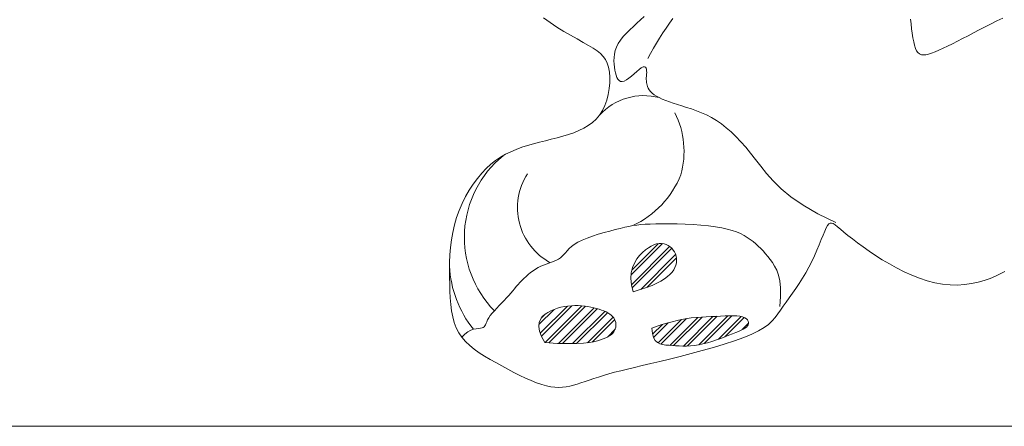
# Model space of a CAD drawing. Units: inches. Extents: x -17 to 1735, y -531 to 60.
# Tile 7 of 27: x 1734.668631 to 1734.675388, y -150.224179 to -150.221388. Entities that reach past the tile are written whole.
import ezdxf

# ---------------------------------------------------------------- set-up
doc = ezdxf.new("R2010")
doc.units = ezdxf.units.IN
doc.header["$MEASUREMENT"] = 0
doc.layers.add('A-FURN', color=242, linetype='Continuous', lineweight=18, true_color=0xcd2027)

# ---------------------------------------------------------------- blocks, each defined once
blk = doc.blocks.new('childrens_room_2')
for p, q in [((70.09560985742021, 54.02979216459647), (70.09445746645682, 54.03061162945817)), ((70.11141095916858, 54.03028320464222), (70.11203336932115, 54.03085697882346)), ((70.11702802801622, 54.03048828868344), (70.11644430215122, 54.02968633954009)), ((70.15854766663281, 54.02956733155446), (70.15844540531864, 54.03041195851841)), ((70.17456501944574, 54.03058353331147), (70.17352318415536, 54.03007965674482)), ((70.09680749046268, 54.02901020311986), (70.09560985742021, 54.02979216459647)), ((70.09801667475725, 54.02827055314123), (70.09680749046268, 54.02901020311986)), ((70.10951143574087, 54.02853423031633), (70.11013384589344, 54.02912183038137)), ((70.11013384589344, 54.02912183038137), (70.11077240256012, 54.02970482181848)), ((70.11077240256012, 54.02970482181848), (70.11141095916858, 54.03028320464222)), ((70.11585971132038, 54.02885184196787), (70.115280310401, 54.0279914208499)), ((70.11644430215122, 54.02968633954009), (70.11585971132038, 54.02885184196787)), ((70.15864992794698, 54.02873307398698), (70.15854766663281, 54.02956733155446)), ((70.15875680256752, 54.02792589209861), (70.15864992794698, 54.02873307398698)), ((70.17145796674188, 54.02904886050095), (70.17044381123154, 54.02853115807232)), ((70.17248596217135, 54.02956656293685), (70.17145796674188, 54.02904886050095)), ((70.17352318415536, 54.03007965674482), (70.17248596217135, 54.02956656293685)), ((70.09920371930232, 54.02757802278796), (70.09801667475725, 54.02827055314123)), ((70.10033493315453, 54.02693742018749), (70.09920371930232, 54.02757802278796)), ((70.10137662531227, 54.02635355346723), (70.10033493315453, 54.02693742018749)), ((70.10790254979977, 54.02674377838997), (70.10837964120904, 54.02734520431699)), ((70.10837964120904, 54.02734520431699), (70.1089213186747, 54.02794202162334)), ((70.1089213186747, 54.02794202162334), (70.10951143574087, 54.02853423031633)), ((70.11471215444502, 54.02711170109109), (70.11416129827151, 54.02621930758908)), ((70.115280310401, 54.0279914208499), (70.11471215444502, 54.02711170109109)), ((70.15887290380081, 54.02716249216467), (70.15875680256752, 54.02792589209861)), ((70.15900284489501, 54.02645958046054), (70.15887290380081, 54.02716249216467)), ((70.16753061291413, 54.02702432905647), (70.1666186226171, 54.02655405706031)), ((70.16847547296086, 54.02751418771225), (70.16753061291413, 54.02702432905647)), ((70.16944810888847, 54.02801806426436), (70.16847547296086, 54.02751418771225)), ((70.17044381123154, 54.02853115807232), (70.16944810888847, 54.02801806426436)), ((70.10230168258889, 54.02582674315493), (70.10137662531227, 54.02635355346723)), ((70.1031093028246, 54.02533935947435), (70.10230168258889, 54.02582674315493)), ((70.10380526161637, 54.02486928504226), (70.1031093028246, 54.02533935947435)), ((70.10698488908704, 54.02491799376588), (70.1072022904514, 54.02552786880409)), ((70.1072022904514, 54.02552786880409), (70.10750619107742, 54.02613774385685)), ((70.10750619107742, 54.02613774385685), (70.10790254979977, 54.02674377838997)), ((70.11363379693242, 54.02532086524155), (70.11313570536325, 54.02442299893158)), ((70.11416129827151, 54.02621930758908), (70.11363379693242, 54.02532086524155)), ((70.1591512391565, 54.02583386326154), (70.15900284489501, 54.02645958046054)), ((70.15932269989165, 54.02530204684302), (70.1591512391565, 54.02583386326154)), ((70.15952193650767, 54.0248769969607), (70.15932269989165, 54.02530204684302)), ((70.16413176951349, 54.0253183688896), (70.16340315756273, 54.0249840513847)), ((70.16491401097622, 54.02569531619377), (70.16413176951349, 54.0253183688896)), ((70.16574469198125, 54.02610913251414), (70.16491401097622, 54.02569531619377)), ((70.1666186226171, 54.02655405706031), (70.16574469198125, 54.02610913251414)), ((70.10439533456113, 54.02439440248276), (70.10380526161637, 54.02486928504226)), ((70.10488529725583, 54.0238925944272), (70.10439533456113, 54.02439440248276)), ((70.10528092529742, 54.02334174349238), (70.10488529725583, 54.0238925944272)), ((70.10674788140344, 54.02313445499607), (70.1067680644442, 54.02371667823757)), ((70.1067680644442, 54.02371667823757), (70.10684360704502, 54.02431272737016)), ((70.10684360704502, 54.02431272737016), (70.10698488908704, 54.02491799376588)), ((70.11313570536325, 54.02442299893158), (70.11267307849951, 54.02353233357138)), ((70.1597540428152, 54.02455621726989), (70.15952193650767, 54.0248769969607)), ((70.16002420884209, 54.02433337091355), (70.1597540428152, 54.02455621726989)), ((70.16033762444161, 54.02420212102737), (70.16002420884209, 54.02433337091355)), ((70.16069947964164, 54.02415613074703), (70.16033762444161, 54.02420212102737)), ((70.16111496429542, 54.02418906320821), (70.16069947964164, 54.02415613074703)), ((70.16158926848905, 54.02429458156115), (70.16111496429542, 54.02418906320821)), ((70.16212758213399, 54.02446634892697), (70.16158926848905, 54.02429458156115)), ((70.1627333650936, 54.02469812446947), (70.16212758213399, 54.02446634892697)), ((70.16340315756273, 54.0249840513847), (70.1627333650936, 54.02469812446947)), ((70.10558799422463, 54.02271973231695), (70.10528092529742, 54.02334174349238)), ((70.10581227969263, 54.02200444351769), (70.10558799422463, 54.02271973231695)), ((70.10595843423974, 54.02118193353675), (70.10581227969263, 54.02200444351769)), ((70.10677267792519, 54.02257066626629), (70.10674788140344, 54.02313445499607)), ((70.10683207412833, 54.02202992068345), (70.10677267792519, 54.02257066626629)), ((70.10691569018994, 54.0215168268682), (70.10683207412833, 54.02202992068345)), ((70.1115233118285, 54.02188340510332), (70.11114838574898, 54.02160439111907)), ((70.11183653510992, 54.02205757281484), (70.1115233118285, 54.02188340510332)), ((70.11207584967954, 54.02210308300567), (70.11183653510992, 54.02205757281484)), ((70.11224711821299, 54.02203452967518), (70.11207584967954, 54.02210308300567)), ((70.1123607205914, 54.02187610811092), (70.11224711821299, 54.02203452967518)), ((70.1124270367541, 54.02165201360043), (70.1123607205914, 54.02187610811092)), ((70.10602661828626, 54.02027095405213), (70.10595843423974, 54.02118193353675)), ((70.10601586919395, 54.01929843057445), (70.10602661828626, 54.02027095405213)), ((70.10701574100997, 54.02103724161719), (70.10691569018994, 54.0215168268682)), ((70.1071348217188, 54.02060201440912), (70.10701574100997, 54.02103724161719)), ((70.10727812211147, 54.02022324288413), (70.1071348217188, 54.02060201440912)), ((70.10745083227405, 54.01991302468963), (70.10727812211147, 54.02022324288413)), ((70.10936611740502, 54.02010812341035), (70.10893352517044, 54.01980606627188)), ((70.10982062272844, 54.02047239700772), (70.10936611740502, 54.02010812341035)), ((70.11028031802155, 54.02086547452057), (70.10982062272844, 54.02047239700772)), ((70.11072848004872, 54.02125394341277), (70.11028031802155, 54.02086547452057)), ((70.11114838574898, 54.02160439111907), (70.11072848004872, 54.02125394341277)), ((70.11239013076877, 54.02001134224559), (70.11239243742195, 54.02011359617467)), ((70.11239243742195, 54.02011359617467), (70.11239935732331, 54.02023486068213)), ((70.11239935732331, 54.02023486068213), (70.11241089053104, 54.02038723342997)), ((70.11241089053104, 54.02038723342997), (70.11242703698693, 54.02058281205103)), ((70.11245644652402, 54.0213864414531), (70.1124270367541, 54.02165201360043)), ((70.11242703698693, 54.02058281205103), (70.1124460667593, 54.02082764538358)), ((70.1124460667593, 54.02082764538358), (70.11245932989871, 54.02110358694193)), ((70.11245932989871, 54.02110358694193), (70.11245644652402, 54.0213864414531)), ((70.10592522449909, 54.01829128859247), (70.10601586919395, 54.01929843057445)), ((70.10765814211803, 54.01968345747303), (70.10745083227405, 54.01991302468963)), ((70.10790524161305, 54.01954663888176), (70.10765814211803, 54.01968345747303)), ((70.10819732067058, 54.01951466656322), (70.10790524161305, 54.01954663888176)), ((70.10853956926033, 54.01959963815028), (70.10819732067058, 54.01951466656322)), ((70.10893352517044, 54.01980606627188), (70.10853956926033, 54.01959963815028)), ((70.11239243742195, 54.01991600125478), (70.11239013076877, 54.02001134224559)), ((70.11239935732331, 54.01981547555482), (70.11239243742195, 54.01991600125478)), ((70.11241089053104, 54.01969766749829), (70.11239935732331, 54.01981547555482)), ((70.11242703698693, 54.01955047943051), (70.11241089053104, 54.01969766749829)), ((70.11244914227748, 54.01936498214348), (70.11242703698693, 54.01955047943051)), ((70.11248393416057, 54.01914492013606), (70.11244914227748, 54.01936498214348)), ((70.11253948580591, 54.0188972063683), (70.11248393416057, 54.01914492013606)), ((70.11262387049968, 54.0186287537785), (70.11253948580591, 54.0188972063683)), ((70.11274516164443, 54.01834647529762), (70.11262387049968, 54.0186287537785)), ((70.11291143229349, 54.01805728388575), (70.11274516164443, 54.01834647529762)), ((70.10550039763214, 54.01628085112173), (70.10575372144697, 54.01727645360955)), ((70.10575372144697, 54.01727645360955), (70.10592522449909, 54.01829128859247)), ((70.11313075584943, 54.01776809246661), (70.11291143229349, 54.01805728388575)), ((70.1134112055984, 54.01748581400756), (70.11313075584943, 54.01776809246661)), ((70.11375893257674, 54.01721582522299), (70.1134112055984, 54.01748581400756)), ((70.11417239893811, 54.01695735801189), (70.11375893257674, 54.01721582522299)), ((70.11464814476088, 54.01670810806393), (70.11417239893811, 54.01695735801189)), ((70.11518271012349, 54.01646577106152), (70.11464814476088, 54.01670810806393)), ((70.10474443692831, 54.0144550456302), (70.10516429029988, 54.01533140662508)), ((70.10516429029988, 54.01533140662508), (70.10550039763214, 54.01628085112173)), ((70.11577263504617, 54.01622804269431), (70.11518271012349, 54.01646577106152)), ((70.11641445949093, 54.01599261863743), (70.11577263504617, 54.01622804269431)), ((70.11710472353619, 54.01575719458055), (70.11641445949093, 54.01599261863743)), ((70.11783996720217, 54.01551946620606), (70.11710472353619, 54.01575719458055)), ((70.11861615390401, 54.01527607306201), (70.11783996720217, 54.01551946620606)), ((70.11942694028724, 54.01501943010811), (70.11861615390401, 54.01527607306201)), ((70.1202654064505, 54.01474089617699), (70.11942694028724, 54.01501943010811)), ((70.10365862586652, 54.01298183595503), (70.10424099793775, 54.013672763604)), ((70.10424099793775, 54.013672763604), (70.10474443692831, 54.0144550456302)), ((70.12112463237602, 54.01443183008672), (70.1202654064505, 54.01474089617699)), ((70.12199769822067, 54.01408359066994), (70.12112463237602, 54.01443183008672)), ((70.12287768390846, 54.01368753674472), (70.12199769822067, 54.01408359066994)), ((70.12375766959624, 54.01323502713643), (70.12287768390846, 54.01368753674472)), ((70.12463073538268, 54.01271742067041), (70.12375766959624, 54.01323502713643)), ((70.10149566713838, 54.01137063301433), (70.1022801848699, 54.01183942527717)), ((70.1022801848699, 54.01183942527717), (70.1030030963116, 54.0123736080481)), ((70.1030030963116, 54.0123736080481), (70.10365862586652, 54.01298183595503)), ((70.125491739203, 54.0121275163678), (70.12463073538268, 54.01271742067041)), ((70.12634265144473, 54.01146387403281), (70.125491739203, 54.0121275163678)), ((70.09685497959029, 54.00970461757828), (70.09785752604833, 54.0099762766244)), ((70.09785752604833, 54.0099762766244), (70.09883023188334, 54.01027005306099)), ((70.09883023188334, 54.01027005306099), (70.09976491507726, 54.01059460152322)), ((70.09976491507726, 54.01059460152322), (70.10065531871399, 54.01095857663171)), ((70.10065531871399, 54.01095857663171), (70.10149566713838, 54.01137063301433)), ((70.1271872203902, 54.01072649366546), (70.12634265144473, 54.01146387403281)), ((70.12802919432173, 54.00991537525118), (70.1271872203902, 54.01072649366546)), ((70.12887232157985, 54.00903051880454), (70.12802919432173, 54.00991537525118)), ((70.08972773888266, 54.00769562276986), (70.09069819871686, 54.00805446920134)), ((70.09069819871686, 54.00805446920134), (70.09169785737643, 54.00837517114855)), ((70.09169785737643, 54.00837517114855), (70.0927196558437, 54.00866606269705)), ((70.0927196558437, 54.00866606269705), (70.09375493066503, 54.00893579848201)), ((70.09375493066503, 54.00893579848201), (70.0947950185032, 54.00919303313862)), ((70.0947950185032, 54.00919303313862), (70.09583125596285, 54.00944642129474)), ((70.09583125596285, 54.00944642129474), (70.09685497959029, 54.00970461757828)), ((70.1297203505051, 54.00807192431097), (70.12887232157985, 54.00903051880454)), ((70.1305770293798, 54.00703959177048), (70.1297203505051, 54.00807192431097)), ((70.0869915523322, 54.0063209796121), (70.08787537827041, 54.00683560934561)), ((70.08787537827041, 54.00683560934561), (70.08878711961327, 54.00729157993777)), ((70.08878711961327, 54.00729157993777), (70.08972773888266, 54.00769562276986)), ((70.13144610648627, 54.00593352118306), (70.1305770293798, 54.00703959177048)), ((70.08449794073707, 54.00435782187418), (70.08530379617471, 54.00508881723948)), ((70.08530379617471, 54.00508881723948), (70.08613467916032, 54.00574095937049)), ((70.08613467916032, 54.00574095937049), (70.0869915523322, 54.0063209796121)), ((70.13234334399343, 54.00475467267682), (70.13144610648627, 54.00593352118306)), ((70.13333255909268, 54.00350784690676), (70.13234334399343, 54.00475467267682)), ((70.08295890602633, 54.0026350704997), (70.08371615026729, 54.00354124187874)), ((70.08371615026729, 54.00354124187874), (70.08449794073707, 54.00435782187418)), ((70.1344895826874, 54.00219880464868), (70.13333255909268, 54.00350784690676)), ((70.08154452785269, 54.00058424474849), (70.0822324649885, 54.00164619937135)), ((70.0822324649885, 54.00164619937135), (70.08295890602633, 54.0026350704997)), ((70.13589024579736, 54.00083330670025), (70.1344895826874, 54.00219880464868)), ((70.08090279543424, 53.99945882287141), (70.08154452785269, 54.00058424474849)), ((70.13761037950056, 53.99941711383002), (70.13589024579736, 54.00083330670025)), ((70.07978874806898, 53.99705604235208), (70.0803149686067, 53.99827954999494)), ((70.0803149686067, 53.99827954999494), (70.08090279543424, 53.99945882287141)), ((70.13972581470037, 53.99795598683562), (70.13761037950056, 53.99941711383002)), ((70.14231238235836, 53.9964556864856), (70.13972581470037, 53.99795598683562)), ((70.0793318345782, 53.99579791619766), (70.07978874806898, 53.99705604235208)), ((70.14544591349434, 53.99492197357034), (70.14231238235836, 53.9964556864856)), ((70.07865384431673, 53.99321563225242), (70.07895192900789, 53.99451478777923)), ((70.07895192900789, 53.99451478777923), (70.0793318345782, 53.99579791619766)), ((70.11005899346085, 53.99439313914484), (70.109376853226, 53.994265341475)), ((70.11073590094341, 53.99449534974559), (70.11005899346085, 53.99439313914484)), ((70.11144034926431, 53.99457444945295), (70.11073590094341, 53.99449534974559)), ((70.11220511201421, 53.99463291442811), (70.11144034926431, 53.99457444945295)), ((70.11306296266733, 53.99467322085405), (70.11220511201421, 53.99463291442811)), ((70.11404667493073, 53.99469784489923), (70.11306296266733, 53.99467322085405)), ((70.11517745519407, 53.99470843734019), (70.11404667493073, 53.99469784489923)), ((70.11643024127582, 53.99470334739311), (70.11517745519407, 53.99470843734019)), ((70.11776840390988, 53.99468009889682), (70.11643024127582, 53.99470334739311)), ((70.11915531377193, 53.99463621568287), (70.11776840390988, 53.99468009889682)), ((70.12055434159586, 53.99456922158282), (70.11915531377193, 53.99463621568287)), ((70.12192885811558, 53.99447664043549), (70.12055434159586, 53.99456922158282)), ((70.12324223394855, 53.99435599605062), (70.12192885811558, 53.99447664043549)), ((70.1244578398869, 53.99420481228156), (70.12324223394855, 53.99435599605062)), ((70.1439956788777, 53.9944393004975), (70.14376176737599, 53.99402243600929)), ((70.14421611396713, 53.99471095959455), (70.1439956788777, 53.9944393004975)), ((70.14444039943513, 53.99484606791379), (70.14421611396713, 53.99471095959455)), ((70.14468586213073, 53.99485328009763), (70.14444039943513, 53.99484606791379)), ((70.14496982867016, 53.99474125075943), (70.14468586213073, 53.99485328009763)), ((70.14530962601887, 53.99451863454164), (70.14496982867016, 53.99474125075943)), ((70.14572258079309, 53.99419408605758), (70.14530962601887, 53.99451863454164)), ((70.07843084226946, 53.99190686046352), (70.07865384431673, 53.99321563225242)), ((70.10401447164944, 53.99288125594324), (70.1030220381904, 53.99256095912864)), ((70.1050256328995, 53.99318064289258), (70.10401447164944, 53.99288125594324)), ((70.10602495162632, 53.99345609354935), (70.1050256328995, 53.99318064289258)), ((70.10698185745744, 53.99370458148627), (70.10602495162632, 53.99345609354935)), ((70.10786578013679, 53.99392308026875), (70.10698185745744, 53.99370458148627)), ((70.10865670658998, 53.99410948057488), (70.10786578013679, 53.99392308026875)), ((70.109376853226, 53.994265341475), (70.10865670658998, 53.99410948057488)), ((70.12554735470215, 53.99402139249144), (70.1244578398869, 53.99420481228156)), ((70.12651568989853, 53.99380715816954), (70.12554735470215, 53.99402139249144)), ((70.1273760650761, 53.99356431037308), (70.12651568989853, 53.99380715816954)), ((70.12814169983497, 53.99329505013014), (70.1273760650761, 53.99356431037308)), ((70.12882581371699, 53.99300157848341), (70.12814169983497, 53.99329505013014)), ((70.12944162638044, 53.992686096461), (70.12882581371699, 53.99300157848341)), ((70.1300023573672, 53.99235080512011), (70.12944162638044, 53.992686096461)), ((70.14320602711408, 53.99276078384577), (70.14287954581553, 53.99195686523166)), ((70.14349978010753, 53.99345700043927), (70.14320602711408, 53.99276078384577)), ((70.14376176737599, 53.99402243600929), (70.14349978010753, 53.99345700043927)), ((70.14622601978365, 53.99377625994242), (70.14572258079309, 53.99419408605758)), ((70.14683325898253, 53.99327445190869), (70.14622601978365, 53.99377625994242)), ((70.14754157101154, 53.99270052199284), (70.14683325898253, 53.99327445190869)), ((70.14834421769368, 53.99206697132325), (70.14754157101154, 53.99270052199284)), ((70.07827329700697, 53.99059424216687), (70.07843084226946, 53.99190686046352)), ((70.09984194546588, 53.99113170618369), (70.0993384074641, 53.99075578729247)), ((70.1004628073529, 53.9915048737734), (70.09984194546588, 53.99113170618369)), ((70.10121563572787, 53.99186974162006), (70.1004628073529, 53.9915048737734)), ((70.10207890277846, 53.99222277887606), (70.10121563572787, 53.99186974162006)), ((70.1030220381904, 53.99256095912864), (70.10207890277846, 53.99222277887606)), ((70.10973540415173, 53.98580639473078), (70.11519221665688, 53.99126320725049)), ((70.10988076387324, 53.98665095893233), (70.11447461730452, 53.99124481239272)), ((70.11324601784465, 53.99083853245105), (70.1137264674285, 53.99105439465933)), ((70.1137264674285, 53.99105439465933), (70.11419259577409, 53.99119817289323)), ((70.11419259577409, 53.99119817289323), (70.11464192422457, 53.99127248088047)), ((70.11464192422457, 53.99127248088047), (70.11507197412313, 53.99127993234873)), ((70.11507197412313, 53.99127993234873), (70.11548026675476, 53.991223141033)), ((70.11548026675476, 53.991223141033), (70.11586418574328, 53.99110533969945)), ((70.11586418574328, 53.99110533969945), (70.11622056395164, 53.99093223728272)), ((70.11622056395164, 53.99093223728272), (70.11654609646533, 53.99071016177771)), ((70.13052122633556, 53.99199790548158), (70.1300023573672, 53.99235080512011)), ((70.13100993814763, 53.99162900247614), (70.13052122633556, 53.99199790548158)), ((70.13147413859726, 53.99124331657225), (70.13100993814763, 53.99162900247614)), ((70.1319179588568, 53.9908394721046), (70.13147413859726, 53.99124331657225)), ((70.1425193735154, 53.99106832360707), (70.1421245476918, 53.99011823798213)), ((70.14287954581553, 53.99195686523166), (70.1425193735154, 53.99106832360707)), ((70.14923446079368, 53.99138630102829), (70.14834421769368, 53.99206697132325)), ((70.15020556225093, 53.99067101222903), (70.14923446079368, 53.99138630102829)), ((70.07811607252691, 53.98798054506045), (70.07817158237916, 53.98928354711682)), ((70.07817158237916, 53.98928354711682), (70.07827329700697, 53.99059424216687)), ((70.09802379239002, 53.98934565578969), (70.09775159730228, 53.98904677320246)), ((70.09829488583958, 53.98967205134835), (70.09802379239002, 53.98934565578969)), ((70.09858856275562, 53.99001990701657), (70.09829488583958, 53.98967205134835)), ((70.09892850830104, 53.99038316994705), (70.09858856275562, 53.99001990701657)), ((70.0993384074641, 53.99075578729247), (70.09892850830104, 53.99038316994705)), ((70.10978827638203, 53.98408874543969), (70.11646500952659, 53.99076547859881)), ((70.1099288537039, 53.9835301183179), (70.11684054317767, 53.99044180774075)), ((70.11075279309765, 53.98858501390936), (70.11123521656148, 53.98920178586417)), ((70.11123521656148, 53.98920178586417), (70.11174352834817, 53.98973230468112)), ((70.11143559102086, 53.98326633406253), (70.1175117062626, 53.98934244934065)), ((70.11174352834817, 53.98973230468112), (70.11225206964767, 53.99018010119329)), ((70.11225206964767, 53.99018010119329), (70.11275372573758, 53.9905479725407)), ((70.11275372573758, 53.9905479725407), (70.11324601784465, 53.99083853245105)), ((70.11654609646533, 53.99071016177771), (70.11683747836972, 53.99044544116481)), ((70.11683747836972, 53.99044544116481), (70.11709140469203, 53.99014440342438)), ((70.11709140469203, 53.99014440342438), (70.11730457063416, 53.98981337654408)), ((70.11730457063416, 53.98981337654408), (70.11747367122328, 53.989458688497)), ((70.11747367122328, 53.989458688497), (70.11759540160304, 53.98908666727805)), ((70.13234553004034, 53.9904160934297), (70.1319179588568, 53.9908394721046)), ((70.1327609833202, 53.98997180489681), (70.13234553004034, 53.9904160934297)), ((70.13316844969405, 53.98950523084789), (70.1327609833202, 53.98997180489681)), ((70.13357206039248, 53.9890149956322), (70.13316844969405, 53.98950523084789)), ((70.1421245476918, 53.99011823798213), (70.14169410570642, 53.98912968735243)), ((70.15125078377199, 53.98993360606112), (70.15020556225093, 53.99067101222903)), ((70.15236338723801, 53.98918658363839), (70.15125078377199, 53.98993360606112)), ((70.15353663441377, 53.98844244610376), (70.15236338723801, 53.98918658363839)), ((70.07809714141652, 53.98669100577393), (70.07811607252691, 53.98798054506045)), ((70.09447125643376, 53.98750746829176), (70.09399989533588, 53.98730235913394)), ((70.09494619788487, 53.98768864117158), (70.09447125643376, 53.98750746829176)), ((70.0954172835441, 53.98785495706983), (70.09494619788487, 53.98768864117158)), ((70.09587707749918, 53.98801549525382), (70.0954172835441, 53.98785495706983)), ((70.09631814372145, 53.98817933500544), (70.09587707749918, 53.98801549525382)), ((70.096733046124, 53.98835555560657), (70.09631814372145, 53.98817933500544)), ((70.09711434873635, 53.98855323632455), (70.096733046124, 53.98835555560657)), ((70.09745461552987, 53.98878145643397), (70.09711434873635, 53.98855323632455)), ((70.09775159730228, 53.98904677320246), (70.09745461552987, 53.98878145643397)), ((70.10998679081561, 53.98707785359732), (70.11032655289048, 53.9878782745713)), ((70.11032655289048, 53.9878782745713), (70.11075279309765, 53.98858501390936)), ((70.11249624676887, 53.98362778533777), (70.1176516682713, 53.98878320684747)), ((70.11754839821836, 53.9875077895835), (70.11738930399181, 53.9871020649793)), ((70.11764580105547, 53.9879113131596), (70.11754839821836, 53.9875077895835)), ((70.11759540160304, 53.98908666727805), (70.11766654865235, 53.98870295304954)), ((70.11768426648226, 53.98831043465765), (70.11764580105547, 53.9879113131596)), ((70.11766654865235, 53.98870295304954), (70.11768426648226, 53.98831043465765)), ((70.13397594652955, 53.98849972360626), (70.13357206039248, 53.9890149956322)), ((70.13438024768723, 53.98795210185785), (70.13397594652955, 53.98849972360626)), ((70.13476913755179, 53.98734106855994), (70.13438024768723, 53.98795210185785)), ((70.14122708497919, 53.98812575071355), (70.14072252293002, 53.98712950709017)), ((70.14169410570642, 53.98912968735243), (70.14122708497919, 53.98812575071355)), ((70.15476330591947, 53.98771385483127), (70.15353663441377, 53.98844244610376)), ((70.15603425692419, 53.98701411232327), (70.15476330591947, 53.98771385483127)), ((70.07810516301427, 53.98542069898979), (70.07809714141652, 53.98669100577393)), ((70.09182508855477, 53.98587512423404), (70.09143529414315, 53.98553602697797)), ((70.09223140748102, 53.98620184065515), (70.09182508855477, 53.98587512423404)), ((70.09265314922553, 53.98651204930359), (70.09223140748102, 53.98620184065515)), ((70.0930892122083, 53.98680162321983), (70.09265314922553, 53.98651204930359)), ((70.09353849479115, 53.9870664354807), (70.0930892122083, 53.98680162321983)), ((70.09399989533588, 53.98730235913394), (70.09353849479115, 53.9870664354807)), ((70.10968788091444, 53.98518110978915), (70.10976380186506, 53.98618003675659)), ((70.10976380186506, 53.98618003675659), (70.10998679081561, 53.98707785359732)), ((70.11651433202088, 53.9858936953446), (70.11607960018912, 53.9855006725906)), ((70.11687502493035, 53.98629281681355), (70.11651433202088, 53.9858936953446)), ((70.11716576422216, 53.98669634037509), (70.11687502493035, 53.98629281681355)), ((70.11738930399181, 53.9871020649793), (70.11716576422216, 53.98669634037509)), ((70.13512279827731, 53.98662962461679), (70.13476913755179, 53.98734106855994)), ((70.13542141207611, 53.98578077093265), (70.13512279827731, 53.98662962461679)), ((70.1356451610441, 53.9847575084263), (70.13542141207611, 53.98578077093265)), ((70.14018146619085, 53.98616036969037), (70.13961299853284, 53.98522308866671)), ((70.14072252293002, 53.98712950709017), (70.14018146619085, 53.98616036969037)), ((70.15733986156877, 53.98635668131323), (70.15603425692419, 53.98701411232327)), ((70.15867049376132, 53.98575502454917), (70.15733986156877, 53.98635668131323)), ((70.16001652752632, 53.98522260479371), (70.15867049376132, 53.98575502454917)), ((70.17410335556954, 53.985981647193), (70.17325065373328, 53.98557039218434)), ((70.17488193734201, 53.98641405797246), (70.17410335556954, 53.985981647193)), ((70.07813051140286, 53.98417539448423), (70.07810516301427, 53.98542069898979)), ((70.07816725056503, 53.9829607017295), (70.07813051140286, 53.98417539448423)), ((70.09005311214017, 53.98412956421674), (70.0897380451311, 53.98376955703719)), ((70.09037478892017, 53.98448461905212), (70.09005311214017, 53.98412956421674)), ((70.09070968530025, 53.98483719769723), (70.09037478892017, 53.98448461905212)), ((70.0910631258262, 53.98518867581737), (70.09070968530025, 53.98483719769723)), ((70.09143529414315, 53.98553602697797), (70.0910631258262, 53.98518867581737)), ((70.10978932289757, 53.98407735845689), (70.10968788091444, 53.98518110978915)), ((70.11009842269007, 53.9828650685144), (70.10978932289757, 53.98407735845689)), ((70.11423174909899, 53.98435296922838), (70.11339877704043, 53.98397810512546)), ((70.11494904967142, 53.98473113491348), (70.11423174909899, 53.98435296922838)), ((70.11556141975919, 53.98511342757268), (70.11494904967142, 53.98473113491348)), ((70.11607960018912, 53.9855006725906), (70.11556141975919, 53.98511342757268)), ((70.13577422739357, 53.98352283800199), (70.1356451610441, 53.9847575084263)), ((70.13902821311379, 53.98431874836973), (70.13843820291689, 53.98344843315721)), ((70.13961299853284, 53.98522308866671), (70.13902821311379, 53.98431874836973)), ((70.16136833688827, 53.98477288478756), (70.16001652752632, 53.98522260479371)), ((70.16271629581345, 53.98441932728605), (70.16136833688827, 53.98477288478756)), ((70.16405077838456, 53.98417539502992), (70.16271629581345, 53.98441932728605)), ((70.16536247946672, 53.9840502234569), (70.16405077838456, 53.98417539502992)), ((70.16664337728756, 53.98403563876349), (70.16536247946672, 53.9840502234569)), ((70.16788577120634, 53.98411913982858), (70.16664337728756, 53.98403563876349)), ((70.16908196034959, 53.98428822551654), (70.16788577120634, 53.98411913982858)), ((70.17022424396012, 53.98453039472082), (70.16908196034959, 53.98428822551654)), ((70.17130492128084, 53.98483314632034), (70.17022424396012, 53.98453039472082)), ((70.1723162914382, 53.98518397917945), (70.17130492128084, 53.98483314632034)), ((70.17325065373328, 53.98557039218434), (70.1723162914382, 53.98518397917945)), ((70.0782242042583, 53.98178158911327), (70.07816725056503, 53.9829607017295)), ((70.08876640507835, 53.98263505979997), (70.08841167932727, 53.98223048160293)), ((70.08910130140023, 53.98302478099362), (70.08876640507835, 53.98263505979997)), ((70.08942297818022, 53.9834021213523), (70.08910130140023, 53.98302478099362)), ((70.0897380451311, 53.98376955703719), (70.08942297818022, 53.9834021213523)), ((70.11134285480831, 53.98323498015674), (70.11009842269007, 53.9828650685144)), ((70.1124393926107, 53.98360571723464), (70.11134285480831, 53.98323498015674)), ((70.11339877704043, 53.98397810512546), (70.1124393926107, 53.98360571723464)), ((70.13578879322043, 53.98203976057124), (70.13577422739357, 53.98352283800199)), ((70.13785406098353, 53.98261322740149), (70.13728688052973, 53.98181421544581)), ((70.13843820291689, 53.98344843315721), (70.13785406098353, 53.98261322740149)), ((70.07831388631487, 53.98064286477751), (70.0782242042583, 53.98178158911327)), ((70.0784488105087, 53.9795493368278), (70.07831388631487, 53.98064286477751)), ((70.08718886693126, 53.98091531589892), (70.08675151878154, 53.9804561703408)), ((70.08761960536825, 53.98136840860974), (70.08718886693126, 53.98091531589892)), ((70.08803051437602, 53.98180857024129), (70.08761960536825, 53.98136840860974)), ((70.08841167932727, 53.98223048160293), (70.08803051437602, 53.98180857024129)), ((70.1356690407952, 53.98027127705285), (70.13578879322043, 53.98203976057124)), ((70.13674775442225, 53.98105248166979), (70.13624777587714, 53.98032911041667)), ((70.13728688052973, 53.98181421544581), (70.13674775442225, 53.98105248166979)), ((70.07864149055561, 53.97850581339156), (70.0784488105087, 53.9795493368278)), ((70.08553201135831, 53.9791111989893), (70.0852004198928, 53.97869662444867)), ((70.08590987139497, 53.97954723364676), (70.08553201135831, 53.9791111989893)), ((70.08632078034455, 53.97999785017458), (70.08590987139497, 53.97954723364676)), ((70.08675151878154, 53.9804561703408), (70.08632078034455, 53.97999785017458)), ((70.09367630142836, 53.97715647001172), (70.09631409799798, 53.97979426654496)), ((70.09391656367691, 53.97562621074616), (70.09864776291536, 53.98035740994822)), ((70.09407255258294, 53.97825192565363), (70.09481758316863, 53.97899695621021)), ((70.09410779761266, 53.97511824018005), (70.09941583290814, 53.98042627546823)), ((70.09426740843222, 53.97852187102256), (70.09470707470203, 53.97892257449569)), ((70.09470707470203, 53.97892257449569), (70.09521022247966, 53.97926123624933)), ((70.09474940773681, 53.97398932876825), (70.10116572975997, 53.98040565084233)), ((70.09521022247966, 53.97926123624933), (70.09574963234948, 53.97955051222237)), ((70.09541204363225, 53.97395276020546), (70.10179794976605, 53.98033866636836)), ((70.09574963234948, 53.97955051222237), (70.09631534370013, 53.97979480449288)), ((70.09631534370013, 53.97979480449288), (70.09690171067953, 53.97999645167004)), ((70.09690171067953, 53.97999645167004), (70.09750308737742, 53.98015779233396)), ((70.09709474678269, 53.97386494187088), (70.10329127679464, 53.98006147187556)), ((70.09750308737742, 53.98015779233396), (70.09811382799992, 53.98028116510835)), ((70.09777502413957, 53.97384601474044), (70.1038421273802, 53.97991311796653)), ((70.09811382799992, 53.98028116510835), (70.09872828663677, 53.9803689085806)), ((70.09872828663677, 53.9803689085806), (70.09934081737767, 53.98042336135262)), ((70.09934081737767, 53.98042336135262), (70.09994577442879, 53.98044686201905)), ((70.09952440521332, 53.97382487430007), (70.1051466494205, 53.97944711849999)), ((70.09994577442879, 53.98044686201905), (70.10053817742622, 53.98044177211563)), ((70.100228645209, 53.97382990980844), (70.10561564012781, 53.97921690472725)), ((70.10053817742622, 53.98044177211563), (70.10111570842449, 53.98041054489152)), ((70.10111570842449, 53.98041054489152), (70.10167671496632, 53.98035565650065)), ((70.10167671496632, 53.98035565650065), (70.10221954453621, 53.98027958311871)), ((70.10221954453621, 53.98027958311871), (70.1027425447351, 53.98018480092145)), ((70.1027425447351, 53.98018480092145), (70.10324406310568, 53.98007378607729)), ((70.10324406310568, 53.98007378607729), (70.10372244719068, 53.9799490147547)), ((70.10372244719068, 53.9799490147547), (70.1041760445328, 53.9798129631294)), ((70.1041760445328, 53.9798129631294), (70.10460320267478, 53.97966751124335)), ((70.10460320267478, 53.97966751124335), (70.10500226927573, 53.97951215470533)), ((70.10500226927573, 53.97951215470533), (70.10537159176195, 53.97934579299039)), ((70.10537159176195, 53.97934579299039), (70.10570951767616, 53.97916732556627)), ((70.10570951767616, 53.97916732556627), (70.10601439467747, 53.97897565192256)), ((70.10601439467747, 53.97897565192256), (70.10628457019222, 53.97876967153428)), ((70.13534403075349, 53.97899247912431), (70.1348722465441, 53.97836858130762)), ((70.13578983752407, 53.97964402182555), (70.13534403075349, 53.97899247912431)), ((70.13624777587714, 53.98032911041667), (70.13578983752407, 53.97964402182555)), ((70.07890444040416, 53.97751710258893), (70.07864149055561, 53.97850581339156)), ((70.07925017371193, 53.97658801254732), (70.07890444040416, 53.97751710258893)), ((70.08445798851201, 53.97736325442969), (70.08435987437727, 53.97712182815161)), ((70.08457304020295, 53.97764237346422), (70.08445798851201, 53.97736325442969)), ((70.08472361958005, 53.97795835987785), (70.08457304020295, 53.97764237346422)), ((70.08492831665674, 53.9783103882641), (70.08472361958005, 53.97795835987785)), ((70.0852004198928, 53.97869662444867), (70.08492831665674, 53.9783103882641)), ((70.0936446416413, 53.97680031592466), (70.09370465769783, 53.97747546116301)), ((70.09370465769783, 53.97747546116301), (70.09392275801977, 53.97804440638577)), ((70.09392275801977, 53.97804440638577), (70.09426740843222, 53.97852187102256)), ((70.10213270574926, 53.97396344879092), (70.10660830525333, 53.97843904833866)), ((70.10295280506719, 53.97408434363609), (70.10688695760794, 53.97801849616957)), ((70.10628457019222, 53.97876967153428), (70.10651839182131, 53.97854828388375)), ((70.10651839182131, 53.97854828388375), (70.10671420716565, 53.97831038845328)), ((70.10671420716565, 53.97831038845328), (70.10687068495784, 53.97805575594833)), ((70.10687068495784, 53.97805575594833), (70.10698777938845, 53.97778764208346)), ((70.10698777938845, 53.97778764208346), (70.10706576589612, 53.97751017380364)), ((70.10706576589612, 53.97751017380364), (70.1071049198031, 53.97722747805386)), ((70.1071049198031, 53.97722747805386), (70.10710551654805, 53.97694368177184)), ((70.11349224073231, 53.97544407982644), (70.11520565872664, 53.9771574978426)), ((70.11365056591924, 53.97490320053333), (70.11619954580559, 53.97745218039057)), ((70.11445830361802, 53.97394041669617), (70.11854165118305, 53.97802376424664)), ((70.11494659115445, 53.97372949974528), (70.1193936751911, 53.97817658381104)), ((70.11665295391461, 53.9775866136319), (70.11511551071774, 53.9771307694013)), ((70.11650060025161, 53.97351298731376), (70.12138147723047, 53.97839386431446)), ((70.11798852293171, 53.97791644841203), (70.11665295391461, 53.9775866136319)), ((70.1171525266359, 53.97346570924714), (70.12212533935556, 53.97843852197405)), ((70.1191567815363, 53.97814310950201), (70.11798852293171, 53.97791644841203)), ((70.11885447475245, 53.9733971358641), (70.12399988040445, 53.97854254152338)), ((70.12019229337923, 53.97828943268399), (70.1191567815363, 53.97814310950201)), ((70.11956906668959, 53.97341252328482), (70.12474546990009, 53.9785889265317)), ((70.12112962222776, 53.97837825372556), (70.12019229337923, 53.97828943268399)), ((70.12200333184913, 53.97843240839432), (70.12112962222776, 53.97837825372556)), ((70.12156425929744, 53.97363719437129), (70.12660742854817, 53.9786803636511)), ((70.1228479858942, 53.97847473247242), (70.12200333184913, 53.97843240839432)), ((70.12246183004348, 53.9738355606882), (70.12731500040857, 53.9786887310533)), ((70.1236903744389, 53.97852310655292), (70.1228479858942, 53.97847473247242)), ((70.1245261930849, 53.97857559055267), (70.1236903744389, 53.97852310655292)), ((70.12534336356796, 53.97862528922127), (70.1245261930849, 53.97857559055267)), ((70.1250067585602, 53.97460996765443), (70.12893685513293, 53.97854006420534)), ((70.12612980785664, 53.97866530730829), (70.12534336356796, 53.97862528922127)), ((70.12610568305129, 53.9750096876582), (70.12946444838192, 53.97836845301793)), ((70.12687344780309, 53.97868874954878), (70.12612980785664, 53.97866530730829)), ((70.12756220520126, 53.97868872069961), (70.12687344780309, 53.97868874954878)), ((70.12818400201971, 53.97865832550309), (70.12756220520126, 53.97868872069961)), ((70.12872675999417, 53.97859066870154), (70.12818400201971, 53.97865832550309)), ((70.12918109983323, 53.97848123425359), (70.12872675999417, 53.97859066870154)), ((70.12913348748, 53.97626697058007), (70.13022539765691, 53.97735888077153)), ((70.12954843714718, 53.97833502298311), (70.12918109983323, 53.97848123425359)), ((70.1298328861699, 53.97815941489392), (70.12954843714718, 53.97833502298311)), ((70.13003856125172, 53.97796179000437), (70.1298328861699, 53.97815941489392)), ((70.13016957674293, 53.97774952834737), (70.13003856125172, 53.97796179000437)), ((70.13015580905952, 53.97709872294075), (70.13022408635473, 53.97731061478992)), ((70.13023004705202, 53.97753000993401), (70.13016957674293, 53.97774952834737)), ((70.13022408635473, 53.97731061478992), (70.13023004705202, 53.97753000993401)), ((70.13369830989862, 53.97718011632099), (70.13291993947817, 53.97660374714764)), ((70.1343363759329, 53.97776642737738), (70.13369830989862, 53.97718011632099)), ((70.1348722465441, 53.97836858130762), (70.1343363759329, 53.97776642737738)), ((70.0796912043111, 53.9757233513796), (70.07925017371193, 53.97658801254732)), ((70.08023621643545, 53.97492558503876), (70.0796912043111, 53.9757233513796)), ((70.08075632068679, 53.97548886628505), (70.08023651643774, 53.97492600397384)), ((70.081275032087, 53.9758910335135), (70.08075632068679, 53.97548886628505)), ((70.08178194787936, 53.97616143633644), (70.081275032087, 53.9758910335135)), ((70.08226636518842, 53.97632900544562), (70.08178194787936, 53.97616143633644)), ((70.08271758113872, 53.97642267151827), (70.08226636518842, 53.97632900544562)), ((70.08312489291305, 53.97647136523159), (70.08271758113872, 53.97642267151827)), ((70.08347759769416, 53.97650401727736), (70.08312489291305, 53.97647136523159)), ((70.0837649926066, 53.97654955831825), (70.08347759769416, 53.97650401727736)), ((70.08398125694251, 53.97663195970967), (70.0837649926066, 53.97654955831825)), ((70.08414009866422, 53.97675535540333), (70.08398125694251, 53.97663195970967)), ((70.08426010778524, 53.97691892001461), (70.08414009866422, 53.97675535540333)), ((70.08435987437727, 53.97712182815161), (70.08426010778524, 53.97691892001461)), ((70.09377424408333, 53.97600425123386), (70.0936446416413, 53.97680031592466)), ((70.09412499931526, 53.97507254767555), (70.09377424408333, 53.97600425123386)), ((70.10560692032917, 53.9749679374276), (70.1069646151259, 53.97632563220253)), ((70.10653611011686, 53.97564529873347), (70.10630242626533, 53.97542414026833)), ((70.10672738113092, 53.97587911316662), (70.10653611011686, 53.97564529873347)), ((70.10687871796429, 53.97612695921129), (70.10672738113092, 53.97587911316662)), ((70.10699214018997, 53.97638929540557), (70.10687871796429, 53.97612695921129)), ((70.1070678315696, 53.97666291190984), (70.10699214018997, 53.97638929540557)), ((70.10710551654805, 53.97694368177184), (70.1070678315696, 53.97666291190984)), ((70.11511551071774, 53.9771307694013), (70.11334162963206, 53.97652607994536)), ((70.11334162963206, 53.97652607994536), (70.11344867963228, 53.97559289566419)), ((70.11344867963228, 53.97559289566419), (70.11365602562321, 53.97488454895796)), ((70.12678396580625, 53.97527122055766), (70.1274145169987, 53.97552117003073)), ((70.1274145169987, 53.97552117003073), (70.12798022660311, 53.97575002178058)), ((70.12798022660311, 53.97575002178058), (70.12847999787076, 53.97596025715614)), ((70.12847999787076, 53.97596025715614), (70.12891493599048, 53.97615666181668)), ((70.12891493599048, 53.97615666181668), (70.12928614609292, 53.97634402144325)), ((70.12928614609292, 53.97634402144325), (70.12959473325057, 53.97652712169514)), ((70.13078984939378, 53.97545723042134), (70.12937638513861, 53.97487732914891)), ((70.12959473325057, 53.97652712169514), (70.12984180271044, 53.97671074825343)), ((70.12984180271044, 53.97671074825343), (70.13002845960321, 53.97689968677735)), ((70.13002845960321, 53.97689968677735), (70.13015580905952, 53.97709872294075)), ((70.13196315565031, 53.97603141884468), (70.13078984939378, 53.97545723042134)), ((70.13291993947817, 53.97660374714764), (70.13196315565031, 53.97603141884468)), ((70.08087857639067, 53.97418781073651), (70.08023621643545, 53.97492558503876)), ((70.0816078208841, 53.97350078351013), (70.08087857639067, 53.97418781073651)), ((70.09472844151199, 53.97399048582014), (70.09412499931526, 53.97507254767555)), ((70.09691040882493, 53.97387007064975), (70.09472844151199, 53.97399048582014)), ((70.09872663412128, 53.97381953841108), (70.09691040882493, 53.97387007064975)), ((70.10022118269583, 53.97382953469644), (70.09872663412128, 53.97381953841108)), ((70.10143811978517, 53.97389070510548), (70.10022118269583, 53.97382953469644)), ((70.1024215108005, 53.97399369523049), (70.10143811978517, 53.97389070510548)), ((70.10321542097839, 53.97412915066382), (70.1024215108005, 53.97399369523049)), ((70.10386391567184, 53.97428771701965), (70.10321542097839, 53.97412915066382)), ((70.10441106011743, 53.97446003987574), (70.10386391567184, 53.97428771701965)), ((70.10489398847452, 53.97463855317477), (70.10441106011743, 53.97446003987574)), ((70.10532211059356, 53.97482284421716), (70.10489398847452, 53.97463855317477)), ((70.1056979051896, 53.97501428865365), (70.10532211059356, 53.97482284421716)), ((70.10602385086125, 53.97521426212046), (70.1056979051896, 53.97501428865365)), ((70.10630242626533, 53.97542414026833), (70.10602385086125, 53.97521426212046)), ((70.11365602562321, 53.97488454895796), (70.11395159690758, 53.97436835610864)), ((70.11395159690758, 53.97436835610864), (70.11432332290453, 53.97401163339094)), ((70.11432332290453, 53.97401163339094), (70.11475913309144, 53.97378169708685)), ((70.11475913309144, 53.97378169708685), (70.11524695682922, 53.97364586348562)), ((70.12150982867345, 53.97362570305853), (70.122270704665, 53.973786338151)), ((70.122270704665, 53.973786338151), (70.12304928207189, 53.97398685337106)), ((70.12304928207189, 53.97398685337106), (70.12383345445735, 53.97421820841413)), ((70.12383345445735, 53.97421820841413), (70.12461111544283, 53.97447136296836)), ((70.12598048722023, 53.97371979808525), (70.12409551594058, 53.97315494573416)), ((70.12461111544283, 53.97447136296836), (70.12537015859155, 53.97473727671462)), ((70.12537015859155, 53.97473727671462), (70.12609847752495, 53.97500690934833)), ((70.12775702065439, 53.97429605546353), (70.12598048722023, 53.97371979808525)), ((70.12609847752495, 53.97500690934833), (70.12678396580625, 53.97527122055766)), ((70.12937638513861, 53.97487732914891), (70.12775702065439, 53.97429605546353)), ((70.08241348668119, 53.97285525838964), (70.0816078208841, 53.97350078351013)), ((70.08328511043104, 53.97224199042688), (70.08241348668119, 53.97285525838964)), ((70.08421222889913, 53.97165173465186), (70.08328511043104, 53.97224199042688)), ((70.11524695682922, 53.97364586348562), (70.11577472347884, 53.97357144885467)), ((70.11577472347884, 53.97357144885467), (70.11633036240121, 53.97352576948327)), ((70.11633036240121, 53.97352576948327), (70.1169041067001, 53.9734826903645)), ((70.1169041067001, 53.9734826903645), (70.11749540340271, 53.97344227139405)), ((70.11749540340271, 53.97344227139405), (70.11810600339552, 53.97341112118596)), ((70.11810600339552, 53.97341112118596), (70.1187376573321, 53.9733958483543)), ((70.12019518484477, 53.97208501096469), (70.11827728741221, 53.97159270598644)), ((70.1187376573321, 53.9733958483543), (70.11939211609891, 53.97340306151312)), ((70.11939211609891, 53.97340306151312), (70.12007113040775, 53.97343936927649)), ((70.12007113040775, 53.97343936927649), (70.12077645102866, 53.97351138025118)), ((70.12215083809454, 53.97260788711577), (70.12019518484477, 53.97208501096469)), ((70.12077645102866, 53.97351138025118), (70.12150982867345, 53.97362570305853)), ((70.12409551594058, 53.97315494573416), (70.12215083809454, 53.97260788711577)), ((70.08518437879277, 53.97107524609459), (70.08421222889913, 53.97165173465186)), ((70.08619109693566, 53.9705032798069), (70.08518437879277, 53.97107524609459)), ((70.08722176770564, 53.96992990842267), (70.08619109693566, 53.9705032798069)), ((70.11316090968786, 53.97034670939905), (70.11169958365964, 53.97000163608613)), ((70.11474011816202, 53.97072331494422), (70.11316090968786, 53.97034670939905)), ((70.11644587695949, 53.97113736090108), (70.11474011816202, 53.97072331494422)), ((70.11827728741221, 53.97159270598644), (70.11644587695949, 53.97113736090108)), ((70.08826516662842, 53.96936247502748), (70.08722176770564, 53.96992990842267)), ((70.08930991707487, 53.96881164031078), (70.08826516662842, 53.96936247502748)), ((70.09034464218306, 53.96828806496199), (70.08930991707487, 53.96881164031078)), ((70.10685974593392, 53.96881850118228), (70.1058578136249, 53.96854246607694)), ((70.10793622118538, 53.96909652753532), (70.10685974593392, 53.96881850118228)), ((70.10909590725672, 53.96938245334462), (70.10793622118538, 53.96909652753532)), ((70.11034747214174, 53.96968218679688), (70.10909590725672, 53.96938245334462)), ((70.11169958365964, 53.97000163608613), (70.11034747214174, 53.96968218679688)), ((70.09135796526564, 53.96780240967785), (70.09034464218306, 53.96828806496199)), ((70.0923385095189, 53.96736533514053), (70.09135796526564, 53.96780240967785)), ((70.0932748983137, 53.96698750203217), (70.0923385095189, 53.96736533514053)), ((70.0941557548463, 53.96667957106405), (70.0932748983137, 53.96698750203217)), ((70.1010106698482, 53.96696245074275), (70.10033749050811, 53.96674967129223)), ((70.1017117918341, 53.96719673705814), (70.1010106698482, 53.96696245074275)), ((70.10244717851631, 53.96744829293897), (70.1017117918341, 53.96719673705814)), ((70.10322315194529, 53.96771288107851), (70.10244717851631, 53.96744829293897)), ((70.1040460342297, 53.96798626418462), (70.10322315194529, 53.96771288107851)), ((70.10492214742001, 53.96826420495057), (70.1040460342297, 53.96798626418462)), ((70.1058578136249, 53.96854246607694), (70.10492214742001, 53.96826420495057)), ((70.09497331118794, 53.96644937234526), (70.0941557548463, 53.96667957106405)), ((70.09573423444411, 53.96629341377269), (70.09497331118794, 53.96644937234526)), ((70.09644880053705, 53.96620537268467), (70.09573423444411, 53.96629341377269)), ((70.09712728544721, 53.96617892640501), (70.09644880053705, 53.96620537268467)), ((70.09777996509686, 53.96620775226478), (70.09712728544721, 53.96617892640501)), ((70.09841711540824, 53.96628552760233), (70.09777996509686, 53.96620775226478)), ((70.09904901224539, 53.96640592973421), (70.09841711540824, 53.96628552760233)), ((70.09968593164697, 53.96656263599874), (70.09904901224539, 53.96640592973421)), ((70.10033749050811, 53.96674967129223), (70.09968593164697, 53.96656263599874)), ((69.75691338651995, 53.95940168826786), (71.77791338646966, 53.95940168826786))]:
    blk.add_line(p, q)
for centre, radius, start, end in [((70.11194614240551, 54.00661341340896), 0.0104500563138801, 75.01516205944708, 137.5045028051908), ((70.1039223432413, 54.007311357373), 0.0150514413292638, 344.3512011530325, 26.71500120300891), ((70.09900702251937, 53.99236748721017), 0.0183274185195923, 129.160039746924, 224.3878839328332), ((70.10086921120413, 53.99753067068235), 0.0109243837345935, 147.3402754188657, 241.444093323535), ((70.1029457656073, 54.00947484180363), 0.0166750041977606, 295.2507305139499, 338.0856005371377), ((70.09682034166647, 53.98811877757402), 0.0187301083385374, 182.3959175938387, 219.009971220419)]:
    blk.add_arc(centre, radius, start, end)

msp = doc.modelspace()

# ---------------------------------------------------------------- block references
at = {"layer": 'A-FURN', "xscale": 0.0393700787401575, "yscale": 0.0393700787401575, "zscale": 0.0393700787401575}
msp.add_blockref('childrens_room_2', (1731.912600860487, -152.3485650223338), dxfattribs=at)

doc.saveas('drawing.dxf')
